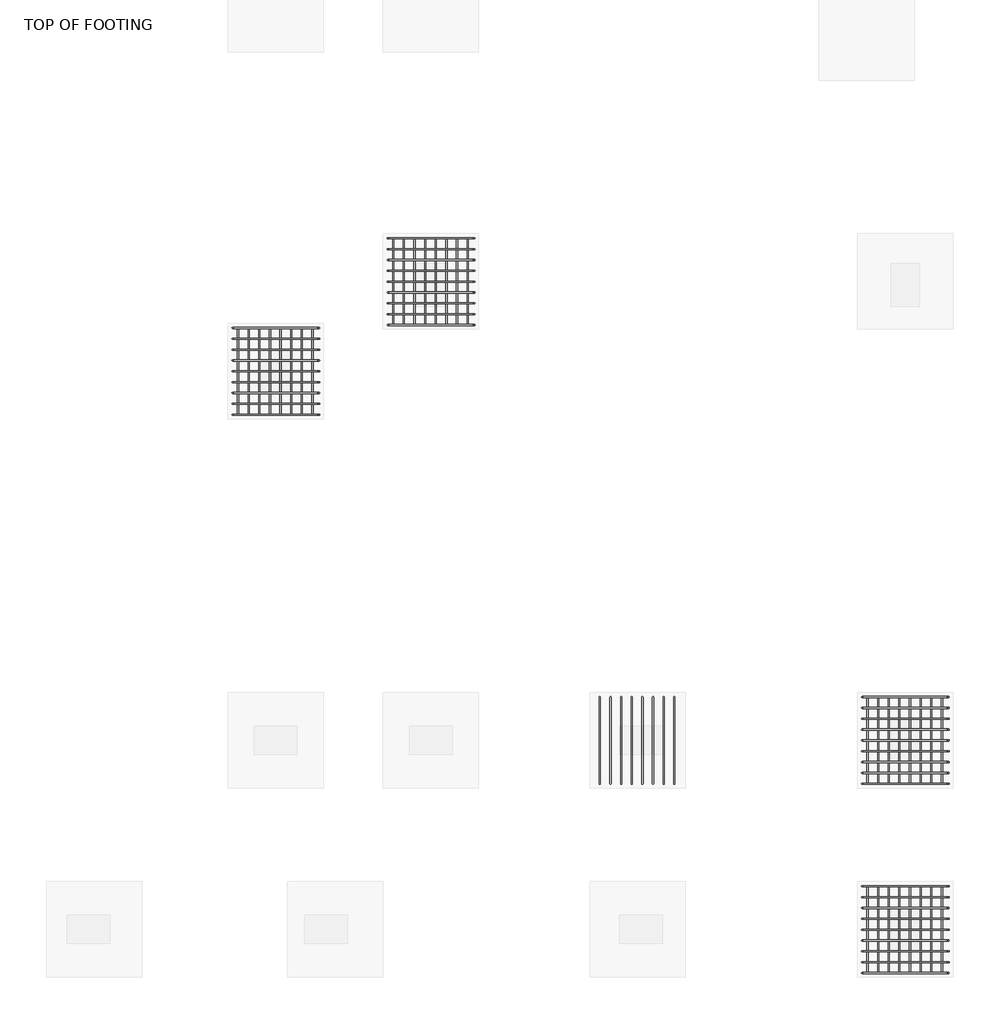
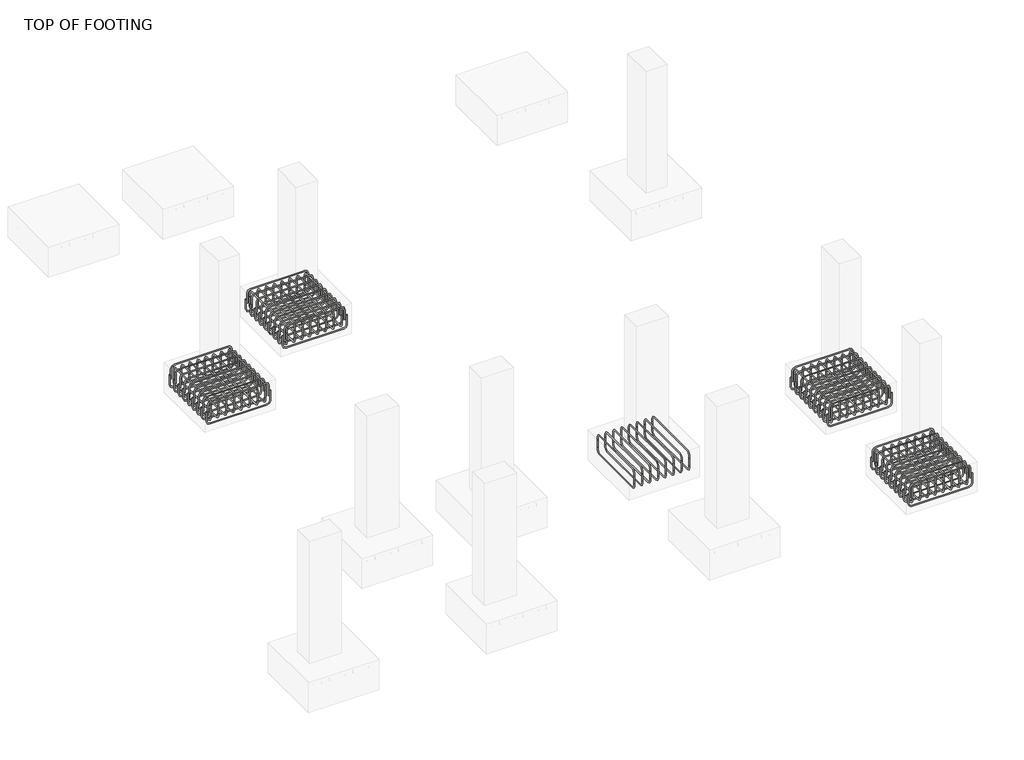
# One storey, part 18 of 20: 18 reinforcing bars.
"""IFC4 building model written with IfcOpenShell, lengths in millimetres."""

from ifc_helpers import new_model, si_unit, point, frame, origin, place, context, project, spatial, polyline, circle_curve, trimmed, segment, composite_curve, source, transform, mapped, element, save
from ifc_brep_helpers import swept_disk

model = new_model("IFC4")

# Units and contexts
model_context = context("Model", 3, world=origin())
ifc_project = project(units=[si_unit("LENGTHUNIT", "METRE", prefix="MILLI")], contexts=[model_context])

# Site, building, storey
site = spatial("IfcSite", under=ifc_project)
building = spatial("IfcBuilding", under=site)
storey = spatial("IfcBuildingStorey", under=building, Name="TOP OF FOOTING", Elevation=-1828.8)

# Reinforcing bars
placement = place(None, origin())
reinforcing_bar_shape = source(origin(), model_context, "Body", "SolidModel", [
    swept_disk(composite_curve([segment(polyline([(8260.5179014, 19241.4849362, -2006.6587682), (8260.5179014, 19241.4849362, -2153.9587682)]), True, "CONTINUOUS"), segment(trimmed(circle_curve(frame((8214.1679014, 19241.4849362, -2153.9587682), z_axis=(0.0, 1.0, 0.0), x_axis=(46.350000000000364, 0.0, 0.0)), 46.35), [point((8260.5179014, 19241.4849362, -2153.9587682))], [point((8214.1679014, 19241.4849362, -2200.3087682))], True, "CARTESIAN"), True, "CONTINUOUS"), segment(polyline([(8214.1679014, 19241.4849362, -2200.3087682), (7399.5679014, 19241.4849362, -2200.3087682)]), True, "CONTINUOUS"), segment(trimmed(circle_curve(frame((7399.5679014, 19241.4849362, -2153.9587682), z_axis=(0.0, 1.0, 0.0), x_axis=(0.0, 0.0, -46.34999999999991)), 46.35), [point((7399.5679014, 19241.4849362, -2200.3087682))], [point((7353.2179014, 19241.4849362, -2153.9587682))], True, "CARTESIAN"), True, "CONTINUOUS"), segment(polyline([(7353.2179014, 19241.4849362, -2153.9587682), (7353.2179014, 19241.4849362, -2006.6587682)]), True, "CONTINUOUS")], self_intersect=False), 6.35),
])
element("IfcReinforcingBar", 1, at=placement, inside=storey, context=model_context, shape_type="MappedRepresentation", body=[
    mapped(reinforcing_bar_shape, transform((0.0, 0.0, 0.0), x_axis=(1.0, 0.0, 0.0), y_axis=(0.0, 1.0, 0.0), z_axis=(0.0, 0.0, 1.0))),
    mapped(reinforcing_bar_shape, transform((0.0, -113.4125, 0.0), x_axis=(1.0, 0.0, 0.0), y_axis=(0.0, 1.0, 0.0), z_axis=(0.0, 0.0, 1.0))),
    mapped(reinforcing_bar_shape, transform((0.0, -226.825, 0.0), x_axis=(1.0, 0.0, 0.0), y_axis=(0.0, 1.0, 0.0), z_axis=(0.0, 0.0, 1.0))),
    mapped(reinforcing_bar_shape, transform((0.0, -340.2375, 0.0), x_axis=(1.0, 0.0, 0.0), y_axis=(0.0, 1.0, 0.0), z_axis=(0.0, 0.0, 1.0))),
    mapped(reinforcing_bar_shape, transform((0.0, -453.65, 0.0), x_axis=(1.0, 0.0, 0.0), y_axis=(0.0, 1.0, 0.0), z_axis=(0.0, 0.0, 1.0))),
    mapped(reinforcing_bar_shape, transform((0.0, -567.0625, 0.0), x_axis=(1.0, 0.0, 0.0), y_axis=(0.0, 1.0, 0.0), z_axis=(0.0, 0.0, 1.0))),
    mapped(reinforcing_bar_shape, transform((0.0, -680.475, 0.0), x_axis=(1.0, 0.0, 0.0), y_axis=(0.0, 1.0, 0.0), z_axis=(0.0, 0.0, 1.0))),
    mapped(reinforcing_bar_shape, transform((0.0, -793.8875, 0.0), x_axis=(1.0, 0.0, 0.0), y_axis=(0.0, 1.0, 0.0), z_axis=(0.0, 0.0, 1.0))),
    mapped(reinforcing_bar_shape, transform((0.0, -907.3, 0.0), x_axis=(1.0, 0.0, 0.0), y_axis=(0.0, 1.0, 0.0), z_axis=(0.0, 0.0, 1.0))),
])
reinforcing_bar_2_shape = source(origin(), model_context, "Body", "SolidModel", [
    swept_disk(composite_curve([segment(polyline([(7372.6920127, 19241.4849362, -2068.8), (7372.6920127, 19241.4849362, -1921.5)]), True, "CONTINUOUS"), segment(trimmed(circle_curve(frame((7419.0420127, 19241.4849362, -1921.5), z_axis=(0.0, 1.0, 0.0), x_axis=(-46.349999999999454, 0.0, 0.0)), 46.35), [point((7372.6920127, 19241.4849362, -1921.5))], [point((7419.0420127, 19241.4849362, -1875.15))], True, "CARTESIAN"), True, "CONTINUOUS"), segment(polyline([(7419.0420127, 19241.4849362, -1875.15), (8188.5054124, 19241.4849362, -1875.15)]), True, "CONTINUOUS"), segment(trimmed(circle_curve(frame((8188.5054124, 19241.4849362, -1921.5), z_axis=(0.0, 1.0, 0.0), x_axis=(0.0, 0.0, 46.34999999999991)), 46.35), [point((8188.5054124, 19241.4849362, -1875.15))], [point((8234.8554124, 19241.4849362, -1921.5))], True, "CARTESIAN"), True, "CONTINUOUS"), segment(polyline([(8234.8554124, 19241.4849362, -1921.5), (8234.8554124, 19241.4849362, -2068.8)]), True, "CONTINUOUS")], self_intersect=False), 6.35),
])
element("IfcReinforcingBar", 2, at=placement, inside=storey, context=model_context, shape_type="MappedRepresentation", body=[
    mapped(reinforcing_bar_2_shape, transform((0.0, 0.0, 0.0), x_axis=(1.0, 0.0, 0.0), y_axis=(0.0, 1.0, 0.0), z_axis=(0.0, 0.0, 1.0))),
    mapped(reinforcing_bar_2_shape, transform((0.0, -113.4125, 0.0), x_axis=(1.0, 0.0, 0.0), y_axis=(0.0, 1.0, 0.0), z_axis=(0.0, 0.0, 1.0))),
    mapped(reinforcing_bar_2_shape, transform((0.0, -226.825, 0.0), x_axis=(1.0, 0.0, 0.0), y_axis=(0.0, 1.0, 0.0), z_axis=(0.0, 0.0, 1.0))),
    mapped(reinforcing_bar_2_shape, transform((0.0, -340.2375, 0.0), x_axis=(1.0, 0.0, 0.0), y_axis=(0.0, 1.0, 0.0), z_axis=(0.0, 0.0, 1.0))),
    mapped(reinforcing_bar_2_shape, transform((0.0, -453.65, 0.0), x_axis=(1.0, 0.0, 0.0), y_axis=(0.0, 1.0, 0.0), z_axis=(0.0, 0.0, 1.0))),
    mapped(reinforcing_bar_2_shape, transform((0.0, -567.0625, 0.0), x_axis=(1.0, 0.0, 0.0), y_axis=(0.0, 1.0, 0.0), z_axis=(0.0, 0.0, 1.0))),
    mapped(reinforcing_bar_2_shape, transform((0.0, -680.475, 0.0), x_axis=(1.0, 0.0, 0.0), y_axis=(0.0, 1.0, 0.0), z_axis=(0.0, 0.0, 1.0))),
    mapped(reinforcing_bar_2_shape, transform((0.0, -793.8875, 0.0), x_axis=(1.0, 0.0, 0.0), y_axis=(0.0, 1.0, 0.0), z_axis=(0.0, 0.0, 1.0))),
    mapped(reinforcing_bar_2_shape, transform((0.0, -907.3, 0.0), x_axis=(1.0, 0.0, 0.0), y_axis=(0.0, 1.0, 0.0), z_axis=(0.0, 0.0, 1.0))),
])
reinforcing_bar_3_shape = source(origin(), model_context, "Body", "SolidModel", [
    swept_disk(composite_curve([segment(polyline([(8189.02094, 19241.4849362, -2086.1951968), (8189.02094, 19241.4849362, -1938.8951968)]), True, "CONTINUOUS"), segment(trimmed(circle_curve(frame((8189.02094, 19195.1349362, -1938.8951968), z_axis=(1.0, 0.0, 0.0), x_axis=(0.0, 46.349999999998545, 0.0)), 46.35), [point((8189.02094, 19241.4849362, -1938.8951968))], [point((8189.02094, 19195.1349362, -1892.5451968))], True, "CARTESIAN"), True, "CONTINUOUS"), segment(polyline([(8189.02094, 19195.1349362, -1892.5451968), (8189.02094, 18380.5349362, -1892.5451968)]), True, "CONTINUOUS"), segment(trimmed(circle_curve(frame((8189.02094, 18380.5349362, -1938.8951968), z_axis=(1.0, 0.0, 0.0), x_axis=(0.0, 0.0, 46.34999999999991)), 46.35), [point((8189.02094, 18380.5349362, -1892.5451968))], [point((8189.02094, 18334.1849362, -1938.8951968))], True, "CARTESIAN"), True, "CONTINUOUS"), segment(polyline([(8189.02094, 18334.1849362, -1938.8951968), (8189.02094, 18334.1849362, -2086.1951968)]), True, "CONTINUOUS")], self_intersect=False), 6.35),
])
element("IfcReinforcingBar", 3, at=placement, inside=storey, context=model_context, shape_type="MappedRepresentation", body=[
    mapped(reinforcing_bar_3_shape, transform((0.0, 0.0, 0.0), x_axis=(1.0, 0.0, 0.0), y_axis=(0.0, 1.0, 0.0), z_axis=(0.0, 0.0, 1.0))),
    mapped(reinforcing_bar_3_shape, transform((-111.2862402, 0.0, 0.0), x_axis=(1.0, 0.0, 0.0), y_axis=(0.0, 1.0, 0.0), z_axis=(0.0, 0.0, 1.0))),
    mapped(reinforcing_bar_3_shape, transform((-222.5724804, 0.0, 0.0), x_axis=(1.0, 0.0, 0.0), y_axis=(0.0, 1.0, 0.0), z_axis=(0.0, 0.0, 1.0))),
    mapped(reinforcing_bar_3_shape, transform((-333.8587205, 0.0, 0.0), x_axis=(1.0, 0.0, 0.0), y_axis=(0.0, 1.0, 0.0), z_axis=(0.0, 0.0, 1.0))),
    mapped(reinforcing_bar_3_shape, transform((-445.1449607, 0.0, 0.0), x_axis=(1.0, 0.0, 0.0), y_axis=(0.0, 1.0, 0.0), z_axis=(0.0, 0.0, 1.0))),
    mapped(reinforcing_bar_3_shape, transform((-556.4312009, 0.0, 0.0), x_axis=(1.0, 0.0, 0.0), y_axis=(0.0, 1.0, 0.0), z_axis=(0.0, 0.0, 1.0))),
    mapped(reinforcing_bar_3_shape, transform((-667.7174411, 0.0, 0.0), x_axis=(1.0, 0.0, 0.0), y_axis=(0.0, 1.0, 0.0), z_axis=(0.0, 0.0, 1.0))),
    mapped(reinforcing_bar_3_shape, transform((-779.0036813, 0.0, 0.0), x_axis=(1.0, 0.0, 0.0), y_axis=(0.0, 1.0, 0.0), z_axis=(0.0, 0.0, 1.0))),
])
reinforcing_bar_4_shape = source(origin(), model_context, "Body", "SolidModel", [
    swept_disk(composite_curve([segment(polyline([(7410.0172587, 19241.4849362, -1979.1645013), (7410.0172587, 19241.4849362, -2126.4645013)]), True, "CONTINUOUS"), segment(trimmed(circle_curve(frame((7410.0172587, 19195.1349362, -2126.4645013), z_axis=(-1.0, 0.0, 0.0), x_axis=(0.0, 46.349999999998545, 0.0)), 46.35), [point((7410.0172587, 19241.4849362, -2126.4645013))], [point((7410.0172587, 19195.1349362, -2172.8145013))], True, "CARTESIAN"), True, "CONTINUOUS"), segment(polyline([(7410.0172587, 19195.1349362, -2172.8145013), (7410.0172587, 18380.5349362, -2172.8145013)]), True, "CONTINUOUS"), segment(trimmed(circle_curve(frame((7410.0172587, 18380.5349362, -2126.4645013), z_axis=(-1.0, 0.0, 0.0), x_axis=(0.0, 0.0, -46.34999999999991)), 46.35), [point((7410.0172587, 18380.5349362, -2172.8145013))], [point((7410.0172587, 18334.1849362, -2126.4645013))], True, "CARTESIAN"), True, "CONTINUOUS"), segment(polyline([(7410.0172587, 18334.1849362, -2126.4645013), (7410.0172587, 18334.1849362, -1979.1645013)]), True, "CONTINUOUS")], self_intersect=False), 6.35),
])
element("IfcReinforcingBar", 4, at=placement, inside=storey, context=model_context, shape_type="MappedRepresentation", body=[
    mapped(reinforcing_bar_4_shape, transform((0.0, 0.0, 0.0), x_axis=(1.0, 0.0, 0.0), y_axis=(0.0, 1.0, 0.0), z_axis=(0.0, 0.0, 1.0))),
    mapped(reinforcing_bar_4_shape, transform((111.2862402, 0.0, 0.0), x_axis=(1.0, 0.0, 0.0), y_axis=(0.0, 1.0, 0.0), z_axis=(0.0, 0.0, 1.0))),
    mapped(reinforcing_bar_4_shape, transform((222.5724804, 0.0, 0.0), x_axis=(1.0, 0.0, 0.0), y_axis=(0.0, 1.0, 0.0), z_axis=(0.0, 0.0, 1.0))),
    mapped(reinforcing_bar_4_shape, transform((333.8587205, 0.0, 0.0), x_axis=(1.0, 0.0, 0.0), y_axis=(0.0, 1.0, 0.0), z_axis=(0.0, 0.0, 1.0))),
    mapped(reinforcing_bar_4_shape, transform((445.1449607, 0.0, 0.0), x_axis=(1.0, 0.0, 0.0), y_axis=(0.0, 1.0, 0.0), z_axis=(0.0, 0.0, 1.0))),
    mapped(reinforcing_bar_4_shape, transform((556.4312009, 0.0, 0.0), x_axis=(1.0, 0.0, 0.0), y_axis=(0.0, 1.0, 0.0), z_axis=(0.0, 0.0, 1.0))),
    mapped(reinforcing_bar_4_shape, transform((667.7174411, 0.0, 0.0), x_axis=(1.0, 0.0, 0.0), y_axis=(0.0, 1.0, 0.0), z_axis=(0.0, 0.0, 1.0))),
    mapped(reinforcing_bar_4_shape, transform((779.0036813, 0.0, 0.0), x_axis=(1.0, 0.0, 0.0), y_axis=(0.0, 1.0, 0.0), z_axis=(0.0, 0.0, 1.0))),
])
reinforcing_bar_5_shape = source(origin(), model_context, "Body", "SolidModel", [
    swept_disk(composite_curve([segment(polyline([(6636.1748054, 18303.3648651, -2006.6587682), (6636.1748054, 18303.3648651, -2153.9587682)]), True, "CONTINUOUS"), segment(trimmed(circle_curve(frame((6589.8248054, 18303.3648651, -2153.9587682), z_axis=(0.0, 1.0, 0.0), x_axis=(46.350000000000364, 0.0, 0.0)), 46.35), [point((6636.1748054, 18303.3648651, -2153.9587682))], [point((6589.8248054, 18303.3648651, -2200.3087682))], True, "CARTESIAN"), True, "CONTINUOUS"), segment(polyline([(6589.8248054, 18303.3648651, -2200.3087682), (5775.2248054, 18303.3648651, -2200.3087682)]), True, "CONTINUOUS"), segment(trimmed(circle_curve(frame((5775.2248054, 18303.3648651, -2153.9587682), z_axis=(0.0, 1.0, 0.0), x_axis=(0.0, 0.0, -46.34999999999991)), 46.35), [point((5775.2248054, 18303.3648651, -2200.3087682))], [point((5728.8748054, 18303.3648651, -2153.9587682))], True, "CARTESIAN"), True, "CONTINUOUS"), segment(polyline([(5728.8748054, 18303.3648651, -2153.9587682), (5728.8748054, 18303.3648651, -2006.6587682)]), True, "CONTINUOUS")], self_intersect=False), 6.35),
])
element("IfcReinforcingBar", 5, at=placement, inside=storey, context=model_context, shape_type="MappedRepresentation", body=[
    mapped(reinforcing_bar_5_shape, transform((0.0, 0.0, 0.0), x_axis=(1.0, 0.0, 0.0), y_axis=(0.0, 1.0, 0.0), z_axis=(0.0, 0.0, 1.0))),
    mapped(reinforcing_bar_5_shape, transform((0.0, -113.4125, 0.0), x_axis=(1.0, 0.0, 0.0), y_axis=(0.0, 1.0, 0.0), z_axis=(0.0, 0.0, 1.0))),
    mapped(reinforcing_bar_5_shape, transform((0.0, -226.825, 0.0), x_axis=(1.0, 0.0, 0.0), y_axis=(0.0, 1.0, 0.0), z_axis=(0.0, 0.0, 1.0))),
    mapped(reinforcing_bar_5_shape, transform((0.0, -340.2375, 0.0), x_axis=(1.0, 0.0, 0.0), y_axis=(0.0, 1.0, 0.0), z_axis=(0.0, 0.0, 1.0))),
    mapped(reinforcing_bar_5_shape, transform((0.0, -453.65, 0.0), x_axis=(1.0, 0.0, 0.0), y_axis=(0.0, 1.0, 0.0), z_axis=(0.0, 0.0, 1.0))),
    mapped(reinforcing_bar_5_shape, transform((0.0, -567.0625, 0.0), x_axis=(1.0, 0.0, 0.0), y_axis=(0.0, 1.0, 0.0), z_axis=(0.0, 0.0, 1.0))),
    mapped(reinforcing_bar_5_shape, transform((0.0, -680.475, 0.0), x_axis=(1.0, 0.0, 0.0), y_axis=(0.0, 1.0, 0.0), z_axis=(0.0, 0.0, 1.0))),
    mapped(reinforcing_bar_5_shape, transform((0.0, -793.8875, 0.0), x_axis=(1.0, 0.0, 0.0), y_axis=(0.0, 1.0, 0.0), z_axis=(0.0, 0.0, 1.0))),
    mapped(reinforcing_bar_5_shape, transform((0.0, -907.3, 0.0), x_axis=(1.0, 0.0, 0.0), y_axis=(0.0, 1.0, 0.0), z_axis=(0.0, 0.0, 1.0))),
])
reinforcing_bar_6_shape = source(origin(), model_context, "Body", "SolidModel", [
    swept_disk(composite_curve([segment(polyline([(5748.3489167, 18303.3648651, -2068.8), (5748.3489167, 18303.3648651, -1921.5)]), True, "CONTINUOUS"), segment(trimmed(circle_curve(frame((5794.6989167, 18303.3648651, -1921.5), z_axis=(0.0, 1.0, 0.0), x_axis=(-46.350000000000364, 0.0, 0.0)), 46.35), [point((5748.3489167, 18303.3648651, -1921.5))], [point((5794.6989167, 18303.3648651, -1875.15))], True, "CARTESIAN"), True, "CONTINUOUS"), segment(polyline([(5794.6989167, 18303.3648651, -1875.15), (6564.1623164, 18303.3648651, -1875.15)]), True, "CONTINUOUS"), segment(trimmed(circle_curve(frame((6564.1623164, 18303.3648651, -1921.5), z_axis=(0.0, 1.0, 0.0), x_axis=(0.0, 0.0, 46.34999999999991)), 46.35), [point((6564.1623164, 18303.3648651, -1875.15))], [point((6610.5123164, 18303.3648651, -1921.5))], True, "CARTESIAN"), True, "CONTINUOUS"), segment(polyline([(6610.5123164, 18303.3648651, -1921.5), (6610.5123164, 18303.3648651, -2068.8)]), True, "CONTINUOUS")], self_intersect=False), 6.35),
])
element("IfcReinforcingBar", 6, at=placement, inside=storey, context=model_context, shape_type="MappedRepresentation", body=[
    mapped(reinforcing_bar_6_shape, transform((0.0, 0.0, 0.0), x_axis=(1.0, 0.0, 0.0), y_axis=(0.0, 1.0, 0.0), z_axis=(0.0, 0.0, 1.0))),
    mapped(reinforcing_bar_6_shape, transform((0.0, -113.4125, 0.0), x_axis=(1.0, 0.0, 0.0), y_axis=(0.0, 1.0, 0.0), z_axis=(0.0, 0.0, 1.0))),
    mapped(reinforcing_bar_6_shape, transform((0.0, -226.825, 0.0), x_axis=(1.0, 0.0, 0.0), y_axis=(0.0, 1.0, 0.0), z_axis=(0.0, 0.0, 1.0))),
    mapped(reinforcing_bar_6_shape, transform((0.0, -340.2375, 0.0), x_axis=(1.0, 0.0, 0.0), y_axis=(0.0, 1.0, 0.0), z_axis=(0.0, 0.0, 1.0))),
    mapped(reinforcing_bar_6_shape, transform((0.0, -453.65, 0.0), x_axis=(1.0, 0.0, 0.0), y_axis=(0.0, 1.0, 0.0), z_axis=(0.0, 0.0, 1.0))),
    mapped(reinforcing_bar_6_shape, transform((0.0, -567.0625, 0.0), x_axis=(1.0, 0.0, 0.0), y_axis=(0.0, 1.0, 0.0), z_axis=(0.0, 0.0, 1.0))),
    mapped(reinforcing_bar_6_shape, transform((0.0, -680.475, 0.0), x_axis=(1.0, 0.0, 0.0), y_axis=(0.0, 1.0, 0.0), z_axis=(0.0, 0.0, 1.0))),
    mapped(reinforcing_bar_6_shape, transform((0.0, -793.8875, 0.0), x_axis=(1.0, 0.0, 0.0), y_axis=(0.0, 1.0, 0.0), z_axis=(0.0, 0.0, 1.0))),
    mapped(reinforcing_bar_6_shape, transform((0.0, -907.3, 0.0), x_axis=(1.0, 0.0, 0.0), y_axis=(0.0, 1.0, 0.0), z_axis=(0.0, 0.0, 1.0))),
])
reinforcing_bar_7_shape = source(origin(), model_context, "Body", "SolidModel", [
    swept_disk(composite_curve([segment(polyline([(6564.677844, 18303.3648651, -2086.1951968), (6564.677844, 18303.3648651, -1938.8951968)]), True, "CONTINUOUS"), segment(trimmed(circle_curve(frame((6564.677844, 18257.0148651, -1938.8951968), z_axis=(1.0, 0.0, 0.0), x_axis=(0.0, 46.349999999998545, 0.0)), 46.35), [point((6564.677844, 18303.3648651, -1938.8951968))], [point((6564.677844, 18257.0148651, -1892.5451968))], True, "CARTESIAN"), True, "CONTINUOUS"), segment(polyline([(6564.677844, 18257.0148651, -1892.5451968), (6564.677844, 17442.4148651, -1892.5451968)]), True, "CONTINUOUS"), segment(trimmed(circle_curve(frame((6564.677844, 17442.4148651, -1938.8951968), z_axis=(1.0, 0.0, 0.0), x_axis=(0.0, 0.0, 46.34999999999991)), 46.35), [point((6564.677844, 17442.4148651, -1892.5451968))], [point((6564.677844, 17396.0648651, -1938.8951968))], True, "CARTESIAN"), True, "CONTINUOUS"), segment(polyline([(6564.677844, 17396.0648651, -1938.8951968), (6564.677844, 17396.0648651, -2086.1951968)]), True, "CONTINUOUS")], self_intersect=False), 6.35),
])
element("IfcReinforcingBar", 7, at=placement, inside=storey, context=model_context, shape_type="MappedRepresentation", body=[
    mapped(reinforcing_bar_7_shape, transform((0.0, 0.0, 0.0), x_axis=(1.0, 0.0, 0.0), y_axis=(0.0, 1.0, 0.0), z_axis=(0.0, 0.0, 1.0))),
    mapped(reinforcing_bar_7_shape, transform((-111.2862402, 0.0, 0.0), x_axis=(1.0, 0.0, 0.0), y_axis=(0.0, 1.0, 0.0), z_axis=(0.0, 0.0, 1.0))),
    mapped(reinforcing_bar_7_shape, transform((-222.5724804, 0.0, 0.0), x_axis=(1.0, 0.0, 0.0), y_axis=(0.0, 1.0, 0.0), z_axis=(0.0, 0.0, 1.0))),
    mapped(reinforcing_bar_7_shape, transform((-333.8587205, 0.0, 0.0), x_axis=(1.0, 0.0, 0.0), y_axis=(0.0, 1.0, 0.0), z_axis=(0.0, 0.0, 1.0))),
    mapped(reinforcing_bar_7_shape, transform((-445.1449607, 0.0, 0.0), x_axis=(1.0, 0.0, 0.0), y_axis=(0.0, 1.0, 0.0), z_axis=(0.0, 0.0, 1.0))),
    mapped(reinforcing_bar_7_shape, transform((-556.4312009, 0.0, 0.0), x_axis=(1.0, 0.0, 0.0), y_axis=(0.0, 1.0, 0.0), z_axis=(0.0, 0.0, 1.0))),
    mapped(reinforcing_bar_7_shape, transform((-667.7174411, 0.0, 0.0), x_axis=(1.0, 0.0, 0.0), y_axis=(0.0, 1.0, 0.0), z_axis=(0.0, 0.0, 1.0))),
    mapped(reinforcing_bar_7_shape, transform((-779.0036813, 0.0, 0.0), x_axis=(1.0, 0.0, 0.0), y_axis=(0.0, 1.0, 0.0), z_axis=(0.0, 0.0, 1.0))),
])
reinforcing_bar_8_shape = source(origin(), model_context, "Body", "SolidModel", [
    swept_disk(composite_curve([segment(polyline([(5785.6741627, 18303.3648651, -1979.1645013), (5785.6741627, 18303.3648651, -2126.4645013)]), True, "CONTINUOUS"), segment(trimmed(circle_curve(frame((5785.6741627, 18257.0148651, -2126.4645013), z_axis=(-1.0, 0.0, 0.0), x_axis=(0.0, 46.349999999998545, 0.0)), 46.35), [point((5785.6741627, 18303.3648651, -2126.4645013))], [point((5785.6741627, 18257.0148651, -2172.8145013))], True, "CARTESIAN"), True, "CONTINUOUS"), segment(polyline([(5785.6741627, 18257.0148651, -2172.8145013), (5785.6741627, 17442.4148651, -2172.8145013)]), True, "CONTINUOUS"), segment(trimmed(circle_curve(frame((5785.6741627, 17442.4148651, -2126.4645013), z_axis=(-1.0, 0.0, 0.0), x_axis=(0.0, 0.0, -46.34999999999991)), 46.35), [point((5785.6741627, 17442.4148651, -2172.8145013))], [point((5785.6741627, 17396.0648651, -2126.4645013))], True, "CARTESIAN"), True, "CONTINUOUS"), segment(polyline([(5785.6741627, 17396.0648651, -2126.4645013), (5785.6741627, 17396.0648651, -1979.1645013)]), True, "CONTINUOUS")], self_intersect=False), 6.35),
])
element("IfcReinforcingBar", 8, at=placement, inside=storey, context=model_context, shape_type="MappedRepresentation", body=[
    mapped(reinforcing_bar_8_shape, transform((0.0, 0.0, 0.0), x_axis=(1.0, 0.0, 0.0), y_axis=(0.0, 1.0, 0.0), z_axis=(0.0, 0.0, 1.0))),
    mapped(reinforcing_bar_8_shape, transform((111.2862402, 0.0, 0.0), x_axis=(1.0, 0.0, 0.0), y_axis=(0.0, 1.0, 0.0), z_axis=(0.0, 0.0, 1.0))),
    mapped(reinforcing_bar_8_shape, transform((222.5724804, 0.0, 0.0), x_axis=(1.0, 0.0, 0.0), y_axis=(0.0, 1.0, 0.0), z_axis=(0.0, 0.0, 1.0))),
    mapped(reinforcing_bar_8_shape, transform((333.8587205, 0.0, 0.0), x_axis=(1.0, 0.0, 0.0), y_axis=(0.0, 1.0, 0.0), z_axis=(0.0, 0.0, 1.0))),
    mapped(reinforcing_bar_8_shape, transform((445.1449607, 0.0, 0.0), x_axis=(1.0, 0.0, 0.0), y_axis=(0.0, 1.0, 0.0), z_axis=(0.0, 0.0, 1.0))),
    mapped(reinforcing_bar_8_shape, transform((556.4312009, 0.0, 0.0), x_axis=(1.0, 0.0, 0.0), y_axis=(0.0, 1.0, 0.0), z_axis=(0.0, 0.0, 1.0))),
    mapped(reinforcing_bar_8_shape, transform((667.7174411, 0.0, 0.0), x_axis=(1.0, 0.0, 0.0), y_axis=(0.0, 1.0, 0.0), z_axis=(0.0, 0.0, 1.0))),
    mapped(reinforcing_bar_8_shape, transform((779.0036813, 0.0, 0.0), x_axis=(1.0, 0.0, 0.0), y_axis=(0.0, 1.0, 0.0), z_axis=(0.0, 0.0, 1.0))),
])
reinforcing_bar_9_shape = source(origin(), model_context, "Body", "SolidModel", [
    swept_disk(composite_curve([segment(polyline([(13222.7663908, 14441.1679708, -2006.6587682), (13222.7663908, 14441.1679708, -2153.9587682)]), True, "CONTINUOUS"), segment(trimmed(circle_curve(frame((13176.4163908, 14441.1679708, -2153.9587682), z_axis=(0.0, 1.0, 0.0), x_axis=(46.350000000000364, 0.0, 0.0)), 46.35), [point((13222.7663908, 14441.1679708, -2153.9587682))], [point((13176.4163908, 14441.1679708, -2200.3087682))], True, "CARTESIAN"), True, "CONTINUOUS"), segment(polyline([(13176.4163908, 14441.1679708, -2200.3087682), (12361.8163908, 14441.1679708, -2200.3087682)]), True, "CONTINUOUS"), segment(trimmed(circle_curve(frame((12361.8163908, 14441.1679708, -2153.9587682), z_axis=(0.0, 1.0, 0.0), x_axis=(0.0, 0.0, -46.34999999999991)), 46.35), [point((12361.8163908, 14441.1679708, -2200.3087682))], [point((12315.4663908, 14441.1679708, -2153.9587682))], True, "CARTESIAN"), True, "CONTINUOUS"), segment(polyline([(12315.4663908, 14441.1679708, -2153.9587682), (12315.4663908, 14441.1679708, -2006.6587682)]), True, "CONTINUOUS")], self_intersect=False), 6.35),
])
element("IfcReinforcingBar", 9, at=placement, inside=storey, context=model_context, shape_type="MappedRepresentation", body=[
    mapped(reinforcing_bar_9_shape, transform((0.0, 0.0, 0.0), x_axis=(1.0, 0.0, 0.0), y_axis=(0.0, 1.0, 0.0), z_axis=(0.0, 0.0, 1.0))),
    mapped(reinforcing_bar_9_shape, transform((0.0, -113.4125, 0.0), x_axis=(1.0, 0.0, 0.0), y_axis=(0.0, 1.0, 0.0), z_axis=(0.0, 0.0, 1.0))),
    mapped(reinforcing_bar_9_shape, transform((0.0, -226.825, 0.0), x_axis=(1.0, 0.0, 0.0), y_axis=(0.0, 1.0, 0.0), z_axis=(0.0, 0.0, 1.0))),
    mapped(reinforcing_bar_9_shape, transform((0.0, -340.2375, 0.0), x_axis=(1.0, 0.0, 0.0), y_axis=(0.0, 1.0, 0.0), z_axis=(0.0, 0.0, 1.0))),
    mapped(reinforcing_bar_9_shape, transform((0.0, -453.65, 0.0), x_axis=(1.0, 0.0, 0.0), y_axis=(0.0, 1.0, 0.0), z_axis=(0.0, 0.0, 1.0))),
    mapped(reinforcing_bar_9_shape, transform((0.0, -567.0625, 0.0), x_axis=(1.0, 0.0, 0.0), y_axis=(0.0, 1.0, 0.0), z_axis=(0.0, 0.0, 1.0))),
    mapped(reinforcing_bar_9_shape, transform((0.0, -680.475, 0.0), x_axis=(1.0, 0.0, 0.0), y_axis=(0.0, 1.0, 0.0), z_axis=(0.0, 0.0, 1.0))),
    mapped(reinforcing_bar_9_shape, transform((0.0, -793.8875, 0.0), x_axis=(1.0, 0.0, 0.0), y_axis=(0.0, 1.0, 0.0), z_axis=(0.0, 0.0, 1.0))),
    mapped(reinforcing_bar_9_shape, transform((0.0, -907.3, 0.0), x_axis=(1.0, 0.0, 0.0), y_axis=(0.0, 1.0, 0.0), z_axis=(0.0, 0.0, 1.0))),
])
reinforcing_bar_10_shape = source(origin(), model_context, "Body", "SolidModel", [
    swept_disk(composite_curve([segment(polyline([(12334.9405021, 14441.1679708, -2068.8), (12334.9405021, 14441.1679708, -1921.5)]), True, "CONTINUOUS"), segment(trimmed(circle_curve(frame((12381.2905021, 14441.1679708, -1921.5), z_axis=(0.0, 1.0, 0.0), x_axis=(-46.350000000000364, 0.0, 0.0)), 46.35), [point((12334.9405021, 14441.1679708, -1921.5))], [point((12381.2905021, 14441.1679708, -1875.15))], True, "CARTESIAN"), True, "CONTINUOUS"), segment(polyline([(12381.2905021, 14441.1679708, -1875.15), (13150.7539017, 14441.1679708, -1875.15)]), True, "CONTINUOUS"), segment(trimmed(circle_curve(frame((13150.7539017, 14441.1679708, -1921.5), z_axis=(0.0, 1.0, 0.0), x_axis=(0.0, 0.0, 46.34999999999991)), 46.35), [point((13150.7539017, 14441.1679708, -1875.15))], [point((13197.1039017, 14441.1679708, -1921.5))], True, "CARTESIAN"), True, "CONTINUOUS"), segment(polyline([(13197.1039017, 14441.1679708, -1921.5), (13197.1039017, 14441.1679708, -2068.8)]), True, "CONTINUOUS")], self_intersect=False), 6.35),
])
element("IfcReinforcingBar", 10, at=placement, inside=storey, context=model_context, shape_type="MappedRepresentation", body=[
    mapped(reinforcing_bar_10_shape, transform((0.0, 0.0, 0.0), x_axis=(1.0, 0.0, 0.0), y_axis=(0.0, 1.0, 0.0), z_axis=(0.0, 0.0, 1.0))),
    mapped(reinforcing_bar_10_shape, transform((0.0, -113.4125, 0.0), x_axis=(1.0, 0.0, 0.0), y_axis=(0.0, 1.0, 0.0), z_axis=(0.0, 0.0, 1.0))),
    mapped(reinforcing_bar_10_shape, transform((0.0, -226.825, 0.0), x_axis=(1.0, 0.0, 0.0), y_axis=(0.0, 1.0, 0.0), z_axis=(0.0, 0.0, 1.0))),
    mapped(reinforcing_bar_10_shape, transform((0.0, -340.2375, 0.0), x_axis=(1.0, 0.0, 0.0), y_axis=(0.0, 1.0, 0.0), z_axis=(0.0, 0.0, 1.0))),
    mapped(reinforcing_bar_10_shape, transform((0.0, -453.65, 0.0), x_axis=(1.0, 0.0, 0.0), y_axis=(0.0, 1.0, 0.0), z_axis=(0.0, 0.0, 1.0))),
    mapped(reinforcing_bar_10_shape, transform((0.0, -567.0625, 0.0), x_axis=(1.0, 0.0, 0.0), y_axis=(0.0, 1.0, 0.0), z_axis=(0.0, 0.0, 1.0))),
    mapped(reinforcing_bar_10_shape, transform((0.0, -680.475, 0.0), x_axis=(1.0, 0.0, 0.0), y_axis=(0.0, 1.0, 0.0), z_axis=(0.0, 0.0, 1.0))),
    mapped(reinforcing_bar_10_shape, transform((0.0, -793.8875, 0.0), x_axis=(1.0, 0.0, 0.0), y_axis=(0.0, 1.0, 0.0), z_axis=(0.0, 0.0, 1.0))),
    mapped(reinforcing_bar_10_shape, transform((0.0, -907.3, 0.0), x_axis=(1.0, 0.0, 0.0), y_axis=(0.0, 1.0, 0.0), z_axis=(0.0, 0.0, 1.0))),
])
reinforcing_bar_11_shape = source(origin(), model_context, "Body", "SolidModel", [
    swept_disk(composite_curve([segment(polyline([(13151.2694294, 14441.1679708, -2086.1951968), (13151.2694294, 14441.1679708, -1938.8951968)]), True, "CONTINUOUS"), segment(trimmed(circle_curve(frame((13151.2694294, 14394.8179708, -1938.8951968), z_axis=(1.0, 0.0, 0.0), x_axis=(0.0, 46.349999999998545, 0.0)), 46.35), [point((13151.2694294, 14441.1679708, -1938.8951968))], [point((13151.2694294, 14394.8179708, -1892.5451968))], True, "CARTESIAN"), True, "CONTINUOUS"), segment(polyline([(13151.2694294, 14394.8179708, -1892.5451968), (13151.2694294, 13580.2179708, -1892.5451968)]), True, "CONTINUOUS"), segment(trimmed(circle_curve(frame((13151.2694294, 13580.2179708, -1938.8951968), z_axis=(1.0, 0.0, 0.0), x_axis=(0.0, 0.0, 46.34999999999991)), 46.35), [point((13151.2694294, 13580.2179708, -1892.5451968))], [point((13151.2694294, 13533.8679708, -1938.8951968))], True, "CARTESIAN"), True, "CONTINUOUS"), segment(polyline([(13151.2694294, 13533.8679708, -1938.8951968), (13151.2694294, 13533.8679708, -2086.1951968)]), True, "CONTINUOUS")], self_intersect=False), 6.35),
])
element("IfcReinforcingBar", 11, at=placement, inside=storey, context=model_context, shape_type="MappedRepresentation", body=[
    mapped(reinforcing_bar_11_shape, transform((0.0, 0.0, 0.0), x_axis=(1.0, 0.0, 0.0), y_axis=(0.0, 1.0, 0.0), z_axis=(0.0, 0.0, 1.0))),
    mapped(reinforcing_bar_11_shape, transform((-111.2862402, 0.0, 0.0), x_axis=(1.0, 0.0, 0.0), y_axis=(0.0, 1.0, 0.0), z_axis=(0.0, 0.0, 1.0))),
    mapped(reinforcing_bar_11_shape, transform((-222.5724804, 0.0, 0.0), x_axis=(1.0, 0.0, 0.0), y_axis=(0.0, 1.0, 0.0), z_axis=(0.0, 0.0, 1.0))),
    mapped(reinforcing_bar_11_shape, transform((-333.8587205, 0.0, 0.0), x_axis=(1.0, 0.0, 0.0), y_axis=(0.0, 1.0, 0.0), z_axis=(0.0, 0.0, 1.0))),
    mapped(reinforcing_bar_11_shape, transform((-445.1449607, 0.0, 0.0), x_axis=(1.0, 0.0, 0.0), y_axis=(0.0, 1.0, 0.0), z_axis=(0.0, 0.0, 1.0))),
    mapped(reinforcing_bar_11_shape, transform((-556.4312009, 0.0, 0.0), x_axis=(1.0, 0.0, 0.0), y_axis=(0.0, 1.0, 0.0), z_axis=(0.0, 0.0, 1.0))),
    mapped(reinforcing_bar_11_shape, transform((-667.7174411, 0.0, 0.0), x_axis=(1.0, 0.0, 0.0), y_axis=(0.0, 1.0, 0.0), z_axis=(0.0, 0.0, 1.0))),
    mapped(reinforcing_bar_11_shape, transform((-779.0036813, 0.0, 0.0), x_axis=(1.0, 0.0, 0.0), y_axis=(0.0, 1.0, 0.0), z_axis=(0.0, 0.0, 1.0))),
])
reinforcing_bar_12_shape = source(origin(), model_context, "Body", "SolidModel", [
    swept_disk(composite_curve([segment(polyline([(12372.2657481, 14441.1679708, -1979.1645013), (12372.2657481, 14441.1679708, -2126.4645013)]), True, "CONTINUOUS"), segment(trimmed(circle_curve(frame((12372.2657481, 14394.8179708, -2126.4645013), z_axis=(-1.0, 0.0, 0.0), x_axis=(0.0, 46.349999999998545, 0.0)), 46.35), [point((12372.2657481, 14441.1679708, -2126.4645013))], [point((12372.2657481, 14394.8179708, -2172.8145013))], True, "CARTESIAN"), True, "CONTINUOUS"), segment(polyline([(12372.2657481, 14394.8179708, -2172.8145013), (12372.2657481, 13580.2179708, -2172.8145013)]), True, "CONTINUOUS"), segment(trimmed(circle_curve(frame((12372.2657481, 13580.2179708, -2126.4645013), z_axis=(-1.0, 0.0, 0.0), x_axis=(0.0, 0.0, -46.34999999999991)), 46.35), [point((12372.2657481, 13580.2179708, -2172.8145013))], [point((12372.2657481, 13533.8679708, -2126.4645013))], True, "CARTESIAN"), True, "CONTINUOUS"), segment(polyline([(12372.2657481, 13533.8679708, -2126.4645013), (12372.2657481, 13533.8679708, -1979.1645013)]), True, "CONTINUOUS")], self_intersect=False), 6.35),
])
element("IfcReinforcingBar", 12, at=placement, inside=storey, context=model_context, shape_type="MappedRepresentation", body=[
    mapped(reinforcing_bar_12_shape, transform((0.0, 0.0, 0.0), x_axis=(1.0, 0.0, 0.0), y_axis=(0.0, 1.0, 0.0), z_axis=(0.0, 0.0, 1.0))),
    mapped(reinforcing_bar_12_shape, transform((111.2862402, 0.0, 0.0), x_axis=(1.0, 0.0, 0.0), y_axis=(0.0, 1.0, 0.0), z_axis=(0.0, 0.0, 1.0))),
    mapped(reinforcing_bar_12_shape, transform((222.5724804, 0.0, 0.0), x_axis=(1.0, 0.0, 0.0), y_axis=(0.0, 1.0, 0.0), z_axis=(0.0, 0.0, 1.0))),
    mapped(reinforcing_bar_12_shape, transform((333.8587205, 0.0, 0.0), x_axis=(1.0, 0.0, 0.0), y_axis=(0.0, 1.0, 0.0), z_axis=(0.0, 0.0, 1.0))),
    mapped(reinforcing_bar_12_shape, transform((445.1449607, 0.0, 0.0), x_axis=(1.0, 0.0, 0.0), y_axis=(0.0, 1.0, 0.0), z_axis=(0.0, 0.0, 1.0))),
    mapped(reinforcing_bar_12_shape, transform((556.4312009, 0.0, 0.0), x_axis=(1.0, 0.0, 0.0), y_axis=(0.0, 1.0, 0.0), z_axis=(0.0, 0.0, 1.0))),
    mapped(reinforcing_bar_12_shape, transform((667.7174411, 0.0, 0.0), x_axis=(1.0, 0.0, 0.0), y_axis=(0.0, 1.0, 0.0), z_axis=(0.0, 0.0, 1.0))),
    mapped(reinforcing_bar_12_shape, transform((779.0036813, 0.0, 0.0), x_axis=(1.0, 0.0, 0.0), y_axis=(0.0, 1.0, 0.0), z_axis=(0.0, 0.0, 1.0))),
])
reinforcing_bar_13_shape = source(origin(), model_context, "Body", "SolidModel", [
    swept_disk(composite_curve([segment(polyline([(13222.7663908, 12461.0575451, -2006.6587682), (13222.7663908, 12461.0575451, -2153.9587682)]), True, "CONTINUOUS"), segment(trimmed(circle_curve(frame((13176.4163908, 12461.0575451, -2153.9587682), z_axis=(0.0, 1.0, 0.0), x_axis=(46.350000000000364, 0.0, 0.0)), 46.35), [point((13222.7663908, 12461.0575451, -2153.9587682))], [point((13176.4163908, 12461.0575451, -2200.3087682))], True, "CARTESIAN"), True, "CONTINUOUS"), segment(polyline([(13176.4163908, 12461.0575451, -2200.3087682), (12361.8163908, 12461.0575451, -2200.3087682)]), True, "CONTINUOUS"), segment(trimmed(circle_curve(frame((12361.8163908, 12461.0575451, -2153.9587682), z_axis=(0.0, 1.0, 0.0), x_axis=(0.0, 0.0, -46.34999999999991)), 46.35), [point((12361.8163908, 12461.0575451, -2200.3087682))], [point((12315.4663908, 12461.0575451, -2153.9587682))], True, "CARTESIAN"), True, "CONTINUOUS"), segment(polyline([(12315.4663908, 12461.0575451, -2153.9587682), (12315.4663908, 12461.0575451, -2006.6587682)]), True, "CONTINUOUS")], self_intersect=False), 6.35),
])
element("IfcReinforcingBar", 13, at=placement, inside=storey, context=model_context, shape_type="MappedRepresentation", body=[
    mapped(reinforcing_bar_13_shape, transform((0.0, 0.0, 0.0), x_axis=(1.0, 0.0, 0.0), y_axis=(0.0, 1.0, 0.0), z_axis=(0.0, 0.0, 1.0))),
    mapped(reinforcing_bar_13_shape, transform((0.0, -113.4125, 0.0), x_axis=(1.0, 0.0, 0.0), y_axis=(0.0, 1.0, 0.0), z_axis=(0.0, 0.0, 1.0))),
    mapped(reinforcing_bar_13_shape, transform((0.0, -226.825, 0.0), x_axis=(1.0, 0.0, 0.0), y_axis=(0.0, 1.0, 0.0), z_axis=(0.0, 0.0, 1.0))),
    mapped(reinforcing_bar_13_shape, transform((0.0, -340.2375, 0.0), x_axis=(1.0, 0.0, 0.0), y_axis=(0.0, 1.0, 0.0), z_axis=(0.0, 0.0, 1.0))),
    mapped(reinforcing_bar_13_shape, transform((0.0, -453.65, 0.0), x_axis=(1.0, 0.0, 0.0), y_axis=(0.0, 1.0, 0.0), z_axis=(0.0, 0.0, 1.0))),
    mapped(reinforcing_bar_13_shape, transform((0.0, -567.0625, 0.0), x_axis=(1.0, 0.0, 0.0), y_axis=(0.0, 1.0, 0.0), z_axis=(0.0, 0.0, 1.0))),
    mapped(reinforcing_bar_13_shape, transform((0.0, -680.475, 0.0), x_axis=(1.0, 0.0, 0.0), y_axis=(0.0, 1.0, 0.0), z_axis=(0.0, 0.0, 1.0))),
    mapped(reinforcing_bar_13_shape, transform((0.0, -793.8875, 0.0), x_axis=(1.0, 0.0, 0.0), y_axis=(0.0, 1.0, 0.0), z_axis=(0.0, 0.0, 1.0))),
    mapped(reinforcing_bar_13_shape, transform((0.0, -907.3, 0.0), x_axis=(1.0, 0.0, 0.0), y_axis=(0.0, 1.0, 0.0), z_axis=(0.0, 0.0, 1.0))),
])
reinforcing_bar_14_shape = source(origin(), model_context, "Body", "SolidModel", [
    swept_disk(composite_curve([segment(polyline([(12334.9405021, 12461.0575451, -2068.8), (12334.9405021, 12461.0575451, -1921.5)]), True, "CONTINUOUS"), segment(trimmed(circle_curve(frame((12381.2905021, 12461.0575451, -1921.5), z_axis=(0.0, 1.0, 0.0), x_axis=(-46.350000000000364, 0.0, 0.0)), 46.35), [point((12334.9405021, 12461.0575451, -1921.5))], [point((12381.2905021, 12461.0575451, -1875.15))], True, "CARTESIAN"), True, "CONTINUOUS"), segment(polyline([(12381.2905021, 12461.0575451, -1875.15), (13150.7539017, 12461.0575451, -1875.15)]), True, "CONTINUOUS"), segment(trimmed(circle_curve(frame((13150.7539017, 12461.0575451, -1921.5), z_axis=(0.0, 1.0, 0.0), x_axis=(0.0, 0.0, 46.34999999999991)), 46.35), [point((13150.7539017, 12461.0575451, -1875.15))], [point((13197.1039017, 12461.0575451, -1921.5))], True, "CARTESIAN"), True, "CONTINUOUS"), segment(polyline([(13197.1039017, 12461.0575451, -1921.5), (13197.1039017, 12461.0575451, -2068.8)]), True, "CONTINUOUS")], self_intersect=False), 6.35),
])
element("IfcReinforcingBar", 14, at=placement, inside=storey, context=model_context, shape_type="MappedRepresentation", body=[
    mapped(reinforcing_bar_14_shape, transform((0.0, 0.0, 0.0), x_axis=(1.0, 0.0, 0.0), y_axis=(0.0, 1.0, 0.0), z_axis=(0.0, 0.0, 1.0))),
    mapped(reinforcing_bar_14_shape, transform((0.0, -113.4125, 0.0), x_axis=(1.0, 0.0, 0.0), y_axis=(0.0, 1.0, 0.0), z_axis=(0.0, 0.0, 1.0))),
    mapped(reinforcing_bar_14_shape, transform((0.0, -226.825, 0.0), x_axis=(1.0, 0.0, 0.0), y_axis=(0.0, 1.0, 0.0), z_axis=(0.0, 0.0, 1.0))),
    mapped(reinforcing_bar_14_shape, transform((0.0, -340.2375, 0.0), x_axis=(1.0, 0.0, 0.0), y_axis=(0.0, 1.0, 0.0), z_axis=(0.0, 0.0, 1.0))),
    mapped(reinforcing_bar_14_shape, transform((0.0, -453.65, 0.0), x_axis=(1.0, 0.0, 0.0), y_axis=(0.0, 1.0, 0.0), z_axis=(0.0, 0.0, 1.0))),
    mapped(reinforcing_bar_14_shape, transform((0.0, -567.0625, 0.0), x_axis=(1.0, 0.0, 0.0), y_axis=(0.0, 1.0, 0.0), z_axis=(0.0, 0.0, 1.0))),
    mapped(reinforcing_bar_14_shape, transform((0.0, -680.475, 0.0), x_axis=(1.0, 0.0, 0.0), y_axis=(0.0, 1.0, 0.0), z_axis=(0.0, 0.0, 1.0))),
    mapped(reinforcing_bar_14_shape, transform((0.0, -793.8875, 0.0), x_axis=(1.0, 0.0, 0.0), y_axis=(0.0, 1.0, 0.0), z_axis=(0.0, 0.0, 1.0))),
    mapped(reinforcing_bar_14_shape, transform((0.0, -907.3, 0.0), x_axis=(1.0, 0.0, 0.0), y_axis=(0.0, 1.0, 0.0), z_axis=(0.0, 0.0, 1.0))),
])
reinforcing_bar_15_shape = source(origin(), model_context, "Body", "SolidModel", [
    swept_disk(composite_curve([segment(polyline([(13151.2694294, 12461.0575451, -2086.1951968), (13151.2694294, 12461.0575451, -1938.8951968)]), True, "CONTINUOUS"), segment(trimmed(circle_curve(frame((13151.2694294, 12414.7075451, -1938.8951968), z_axis=(1.0, 0.0, 0.0), x_axis=(0.0, 46.350000000000364, 0.0)), 46.35), [point((13151.2694294, 12461.0575451, -1938.8951968))], [point((13151.2694294, 12414.7075451, -1892.5451968))], True, "CARTESIAN"), True, "CONTINUOUS"), segment(polyline([(13151.2694294, 12414.7075451, -1892.5451968), (13151.2694294, 11600.1075451, -1892.5451968)]), True, "CONTINUOUS"), segment(trimmed(circle_curve(frame((13151.2694294, 11600.1075451, -1938.8951968), z_axis=(1.0, 0.0, 0.0), x_axis=(0.0, 0.0, 46.34999999999991)), 46.35), [point((13151.2694294, 11600.1075451, -1892.5451968))], [point((13151.2694294, 11553.7575451, -1938.8951968))], True, "CARTESIAN"), True, "CONTINUOUS"), segment(polyline([(13151.2694294, 11553.7575451, -1938.8951968), (13151.2694294, 11553.7575451, -2086.1951968)]), True, "CONTINUOUS")], self_intersect=False), 6.35),
])
element("IfcReinforcingBar", 15, at=placement, inside=storey, context=model_context, shape_type="MappedRepresentation", body=[
    mapped(reinforcing_bar_15_shape, transform((0.0, 0.0, 0.0), x_axis=(1.0, 0.0, 0.0), y_axis=(0.0, 1.0, 0.0), z_axis=(0.0, 0.0, 1.0))),
    mapped(reinforcing_bar_15_shape, transform((-111.2862402, 0.0, 0.0), x_axis=(1.0, 0.0, 0.0), y_axis=(0.0, 1.0, 0.0), z_axis=(0.0, 0.0, 1.0))),
    mapped(reinforcing_bar_15_shape, transform((-222.5724804, 0.0, 0.0), x_axis=(1.0, 0.0, 0.0), y_axis=(0.0, 1.0, 0.0), z_axis=(0.0, 0.0, 1.0))),
    mapped(reinforcing_bar_15_shape, transform((-333.8587205, 0.0, 0.0), x_axis=(1.0, 0.0, 0.0), y_axis=(0.0, 1.0, 0.0), z_axis=(0.0, 0.0, 1.0))),
    mapped(reinforcing_bar_15_shape, transform((-445.1449607, 0.0, 0.0), x_axis=(1.0, 0.0, 0.0), y_axis=(0.0, 1.0, 0.0), z_axis=(0.0, 0.0, 1.0))),
    mapped(reinforcing_bar_15_shape, transform((-556.4312009, 0.0, 0.0), x_axis=(1.0, 0.0, 0.0), y_axis=(0.0, 1.0, 0.0), z_axis=(0.0, 0.0, 1.0))),
    mapped(reinforcing_bar_15_shape, transform((-667.7174411, 0.0, 0.0), x_axis=(1.0, 0.0, 0.0), y_axis=(0.0, 1.0, 0.0), z_axis=(0.0, 0.0, 1.0))),
    mapped(reinforcing_bar_15_shape, transform((-779.0036813, 0.0, 0.0), x_axis=(1.0, 0.0, 0.0), y_axis=(0.0, 1.0, 0.0), z_axis=(0.0, 0.0, 1.0))),
])
reinforcing_bar_16_shape = source(origin(), model_context, "Body", "SolidModel", [
    swept_disk(composite_curve([segment(polyline([(12372.2657481, 12461.0575451, -1979.1645013), (12372.2657481, 12461.0575451, -2126.4645013)]), True, "CONTINUOUS"), segment(trimmed(circle_curve(frame((12372.2657481, 12414.7075451, -2126.4645013), z_axis=(-1.0, 0.0, 0.0), x_axis=(0.0, 46.350000000000364, 0.0)), 46.35), [point((12372.2657481, 12461.0575451, -2126.4645013))], [point((12372.2657481, 12414.7075451, -2172.8145013))], True, "CARTESIAN"), True, "CONTINUOUS"), segment(polyline([(12372.2657481, 12414.7075451, -2172.8145013), (12372.2657481, 11600.1075451, -2172.8145013)]), True, "CONTINUOUS"), segment(trimmed(circle_curve(frame((12372.2657481, 11600.1075451, -2126.4645013), z_axis=(-1.0, 0.0, 0.0), x_axis=(0.0, 0.0, -46.34999999999991)), 46.35), [point((12372.2657481, 11600.1075451, -2172.8145013))], [point((12372.2657481, 11553.7575451, -2126.4645013))], True, "CARTESIAN"), True, "CONTINUOUS"), segment(polyline([(12372.2657481, 11553.7575451, -2126.4645013), (12372.2657481, 11553.7575451, -1979.1645013)]), True, "CONTINUOUS")], self_intersect=False), 6.35),
])
element("IfcReinforcingBar", 16, at=placement, inside=storey, context=model_context, shape_type="MappedRepresentation", body=[
    mapped(reinforcing_bar_16_shape, transform((0.0, 0.0, 0.0), x_axis=(1.0, 0.0, 0.0), y_axis=(0.0, 1.0, 0.0), z_axis=(0.0, 0.0, 1.0))),
    mapped(reinforcing_bar_16_shape, transform((111.2862402, 0.0, 0.0), x_axis=(1.0, 0.0, 0.0), y_axis=(0.0, 1.0, 0.0), z_axis=(0.0, 0.0, 1.0))),
    mapped(reinforcing_bar_16_shape, transform((222.5724804, 0.0, 0.0), x_axis=(1.0, 0.0, 0.0), y_axis=(0.0, 1.0, 0.0), z_axis=(0.0, 0.0, 1.0))),
    mapped(reinforcing_bar_16_shape, transform((333.8587205, 0.0, 0.0), x_axis=(1.0, 0.0, 0.0), y_axis=(0.0, 1.0, 0.0), z_axis=(0.0, 0.0, 1.0))),
    mapped(reinforcing_bar_16_shape, transform((445.1449607, 0.0, 0.0), x_axis=(1.0, 0.0, 0.0), y_axis=(0.0, 1.0, 0.0), z_axis=(0.0, 0.0, 1.0))),
    mapped(reinforcing_bar_16_shape, transform((556.4312009, 0.0, 0.0), x_axis=(1.0, 0.0, 0.0), y_axis=(0.0, 1.0, 0.0), z_axis=(0.0, 0.0, 1.0))),
    mapped(reinforcing_bar_16_shape, transform((667.7174411, 0.0, 0.0), x_axis=(1.0, 0.0, 0.0), y_axis=(0.0, 1.0, 0.0), z_axis=(0.0, 0.0, 1.0))),
    mapped(reinforcing_bar_16_shape, transform((779.0036813, 0.0, 0.0), x_axis=(1.0, 0.0, 0.0), y_axis=(0.0, 1.0, 0.0), z_axis=(0.0, 0.0, 1.0))),
])
reinforcing_bar_17_shape = source(origin(), model_context, "Body", "SolidModel", [
    swept_disk(composite_curve([segment(polyline([(10351.2694294, 14441.1679708, -2086.1951968), (10351.2694294, 14441.1679708, -1938.8951968)]), True, "CONTINUOUS"), segment(trimmed(circle_curve(frame((10351.2694294, 14394.8179708, -1938.8951968), z_axis=(1.0, 0.0, 0.0), x_axis=(0.0, 46.349999999998545, 0.0)), 46.35), [point((10351.2694294, 14441.1679708, -1938.8951968))], [point((10351.2694294, 14394.8179708, -1892.5451968))], True, "CARTESIAN"), True, "CONTINUOUS"), segment(polyline([(10351.2694294, 14394.8179708, -1892.5451968), (10351.2694294, 13580.2179708, -1892.5451968)]), True, "CONTINUOUS"), segment(trimmed(circle_curve(frame((10351.2694294, 13580.2179708, -1938.8951968), z_axis=(1.0, 0.0, 0.0), x_axis=(0.0, 0.0, 46.34999999999991)), 46.35), [point((10351.2694294, 13580.2179708, -1892.5451968))], [point((10351.2694294, 13533.8679708, -1938.8951968))], True, "CARTESIAN"), True, "CONTINUOUS"), segment(polyline([(10351.2694294, 13533.8679708, -1938.8951968), (10351.2694294, 13533.8679708, -2086.1951968)]), True, "CONTINUOUS")], self_intersect=False), 6.35),
])
element("IfcReinforcingBar", 17, at=placement, inside=storey, context=model_context, shape_type="MappedRepresentation", body=[
    mapped(reinforcing_bar_17_shape, transform((0.0, 0.0, 0.0), x_axis=(1.0, 0.0, 0.0), y_axis=(0.0, 1.0, 0.0), z_axis=(0.0, 0.0, 1.0))),
    mapped(reinforcing_bar_17_shape, transform((-111.2862402, 0.0, 0.0), x_axis=(1.0, 0.0, 0.0), y_axis=(0.0, 1.0, 0.0), z_axis=(0.0, 0.0, 1.0))),
    mapped(reinforcing_bar_17_shape, transform((-222.5724804, 0.0, 0.0), x_axis=(1.0, 0.0, 0.0), y_axis=(0.0, 1.0, 0.0), z_axis=(0.0, 0.0, 1.0))),
    mapped(reinforcing_bar_17_shape, transform((-333.8587205, 0.0, 0.0), x_axis=(1.0, 0.0, 0.0), y_axis=(0.0, 1.0, 0.0), z_axis=(0.0, 0.0, 1.0))),
    mapped(reinforcing_bar_17_shape, transform((-445.1449607, 0.0, 0.0), x_axis=(1.0, 0.0, 0.0), y_axis=(0.0, 1.0, 0.0), z_axis=(0.0, 0.0, 1.0))),
    mapped(reinforcing_bar_17_shape, transform((-556.4312009, 0.0, 0.0), x_axis=(1.0, 0.0, 0.0), y_axis=(0.0, 1.0, 0.0), z_axis=(0.0, 0.0, 1.0))),
    mapped(reinforcing_bar_17_shape, transform((-667.7174411, 0.0, 0.0), x_axis=(1.0, 0.0, 0.0), y_axis=(0.0, 1.0, 0.0), z_axis=(0.0, 0.0, 1.0))),
    mapped(reinforcing_bar_17_shape, transform((-779.0036813, 0.0, 0.0), x_axis=(1.0, 0.0, 0.0), y_axis=(0.0, 1.0, 0.0), z_axis=(0.0, 0.0, 1.0))),
])
reinforcing_bar_18_shape = source(origin(), model_context, "Body", "SolidModel", [
    swept_disk(composite_curve([segment(polyline([(9572.2657481, 14441.1679708, -1979.1645013), (9572.2657481, 14441.1679708, -2126.4645013)]), True, "CONTINUOUS"), segment(trimmed(circle_curve(frame((9572.2657481, 14394.8179708, -2126.4645013), z_axis=(-1.0, 0.0, 0.0), x_axis=(0.0, 46.349999999998545, 0.0)), 46.35), [point((9572.2657481, 14441.1679708, -2126.4645013))], [point((9572.2657481, 14394.8179708, -2172.8145013))], True, "CARTESIAN"), True, "CONTINUOUS"), segment(polyline([(9572.2657481, 14394.8179708, -2172.8145013), (9572.2657481, 13580.2179708, -2172.8145013)]), True, "CONTINUOUS"), segment(trimmed(circle_curve(frame((9572.2657481, 13580.2179708, -2126.4645013), z_axis=(-1.0, 0.0, 0.0), x_axis=(0.0, 0.0, -46.34999999999991)), 46.35), [point((9572.2657481, 13580.2179708, -2172.8145013))], [point((9572.2657481, 13533.8679708, -2126.4645013))], True, "CARTESIAN"), True, "CONTINUOUS"), segment(polyline([(9572.2657481, 13533.8679708, -2126.4645013), (9572.2657481, 13533.8679708, -1979.1645013)]), True, "CONTINUOUS")], self_intersect=False), 6.35),
])
element("IfcReinforcingBar", 18, at=placement, inside=storey, context=model_context, shape_type="MappedRepresentation", body=[
    mapped(reinforcing_bar_18_shape, transform((0.0, 0.0, 0.0), x_axis=(1.0, 0.0, 0.0), y_axis=(0.0, 1.0, 0.0), z_axis=(0.0, 0.0, 1.0))),
    mapped(reinforcing_bar_18_shape, transform((111.2862402, 0.0, 0.0), x_axis=(1.0, 0.0, 0.0), y_axis=(0.0, 1.0, 0.0), z_axis=(0.0, 0.0, 1.0))),
    mapped(reinforcing_bar_18_shape, transform((222.5724804, 0.0, 0.0), x_axis=(1.0, 0.0, 0.0), y_axis=(0.0, 1.0, 0.0), z_axis=(0.0, 0.0, 1.0))),
    mapped(reinforcing_bar_18_shape, transform((333.8587205, 0.0, 0.0), x_axis=(1.0, 0.0, 0.0), y_axis=(0.0, 1.0, 0.0), z_axis=(0.0, 0.0, 1.0))),
    mapped(reinforcing_bar_18_shape, transform((445.1449607, 0.0, 0.0), x_axis=(1.0, 0.0, 0.0), y_axis=(0.0, 1.0, 0.0), z_axis=(0.0, 0.0, 1.0))),
    mapped(reinforcing_bar_18_shape, transform((556.4312009, 0.0, 0.0), x_axis=(1.0, 0.0, 0.0), y_axis=(0.0, 1.0, 0.0), z_axis=(0.0, 0.0, 1.0))),
    mapped(reinforcing_bar_18_shape, transform((667.7174411, 0.0, 0.0), x_axis=(1.0, 0.0, 0.0), y_axis=(0.0, 1.0, 0.0), z_axis=(0.0, 0.0, 1.0))),
    mapped(reinforcing_bar_18_shape, transform((779.0036813, 0.0, 0.0), x_axis=(1.0, 0.0, 0.0), y_axis=(0.0, 1.0, 0.0), z_axis=(0.0, 0.0, 1.0))),
])

save(model, "model.ifc")

# Revit data of these elements
# Elements 1, 2, 3, 4, 5, 6, 7, 8, 9, 10, 11, 12, 13, 14, 15, 16, 17, 18 (IfcReinforcingBar)
#   Phase Created = New Construction
